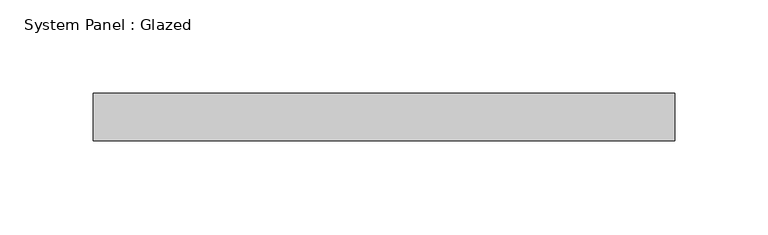
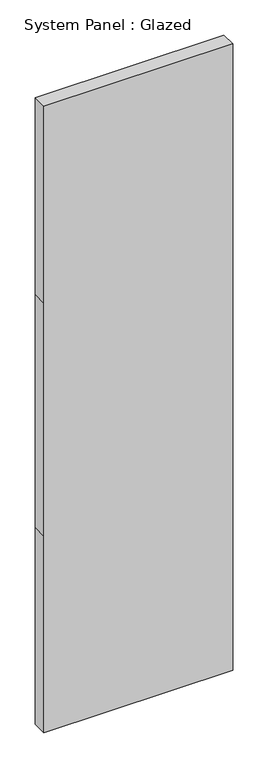
"""IFC4 building model written with IfcOpenShell, lengths in millimetres: plate geometry, System Panel : Glazed."""

from ifc_helpers import new_model, si_unit, frame, origin, place, context, project, spatial, polyline, outline, extrude, source, transform, mapped, element, save


def system_panel_glazed_58042333(model_context):
    return source(origin(), model_context, "Body", "SweptSolid", [
        extrude(outline(polyline([(0.0, -155.575), (0.0, 155.575), (342.9, 155.575), (749.3, 155.575), (1092.2, 155.575), (1092.2, -155.575), (749.3, -155.575), (342.9, -155.575), (0.0, -155.575)])), frame((0.0, 19.05, 0.0), z_axis=(0.0, 1.0, 0.0), x_axis=(0.0, 0.0, 1.0)), (0.0, 0.0, 1.0), 25.4),
    ])


if __name__ == "__main__":
    model = new_model("IFC4")
    model_context = context("Model", 3, world=origin())
    ifc_project = project(units=[si_unit("LENGTHUNIT", "METRE", prefix="MILLI")], contexts=[model_context])
    site = spatial("IfcSite", under=ifc_project)
    building = spatial("IfcBuilding", under=site)
    placement = place(None, origin())
    system_panel_glazed_shape = system_panel_glazed_58042333(model_context)
    element("IfcPlate", 1, ObjectType="System Panel : Glazed", at=placement, inside=building, context=model_context, shape_type="MappedRepresentation", body=[
        mapped(system_panel_glazed_shape, transform((0.0, 0.0, 0.0), x_axis=(1.0, 0.0, 0.0), y_axis=(0.0, 1.0, 0.0), z_axis=(0.0, 0.0, 1.0))),
    ])
    save(model, "model.ifc")

# Revit data of these elements
# Type "System Panel : Glazed"
#   Construction Type Id = "GSP4R"
#   Analytic Construction = "1/8 in Pilkington single glazing"
#   Visual Light Transmittance = 0.9
#   Solar Heat Gain Coefficient = 0.86
#   Heat Transfer Coefficient (U) = 1.18115 BTU/(h·ft²·°F)
#   Define Thermal Properties by = 1
# Element 1 (IfcPlate, "System Panel : Glazed")
#   Materials on its faces: "Glass"
# Materials
#   "Glass": class "Glass", colour RGB 0 128 192, transparency 0.75, Description = "Soda Lime Glass", Cost = 0
